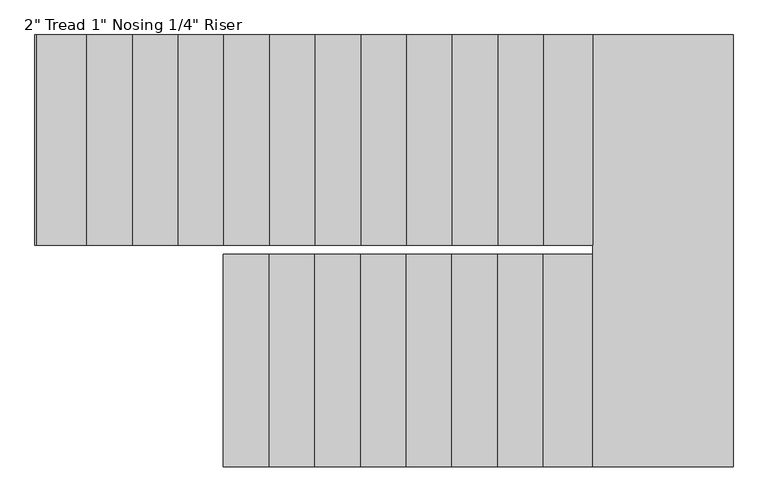
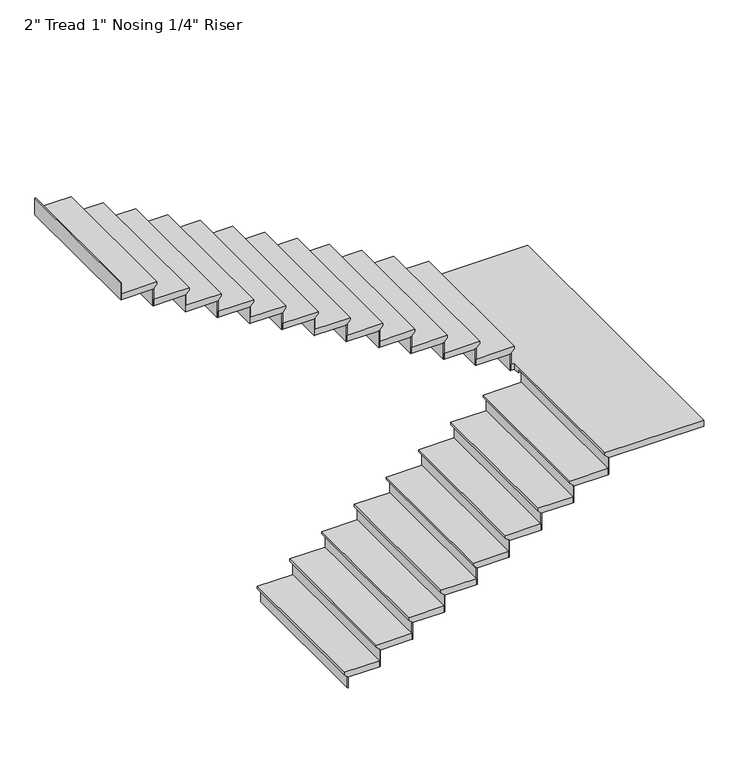
"""IFC4 building model written with IfcOpenShell, lengths in millimetres: stair flight geometry."""

from ifc_helpers import new_model, si_unit, origin, place, context, project, spatial, faceted_brep, source, transform, mapped, element, save


def stair_flight_9b376cb7(model_context):
    return source(origin(), model_context, "Body", "Brep", [
        faceted_brep([(2827.8890963, -935.5037749, 9263.4954545), (2827.8890963, -935.5037749, 9282.5454545), (2827.8890963, 245.5962251, 9282.5454545), (2827.8890963, 245.5962251, 9263.4954545), (2853.2890963, -935.5037749, 9238.0954545), (2853.2890963, 245.5962251, 9238.0954545), (3107.2890963, -935.5037749, 9282.5454545), (3107.2890963, 245.5962251, 9282.5454545), (2853.2890963, 245.5962251, 9231.7454545), (3107.2890963, 245.5962251, 9231.7454545), (3107.2890963, -935.5037749, 9231.7454545), (2853.2890963, -935.5037749, 9231.7454545)], [[[0, 1, 2, 3]], [[4, 0, 3, 5]], [[2, 1, 6, 7]], [[8, 9, 10, 11]], [[2, 7, 9, 8, 5, 3]], [[8, 11, 4, 5]], [[6, 1, 0, 4, 11, 10]], [[7, 6, 10, 9]]]),
        faceted_brep([(2853.2890963, -935.5037749, 9231.7454545), (2853.2890963, -935.5037749, 9144.0), (2859.6390963, -935.5037749, 9144.0), (2859.6390963, -935.5037749, 9231.7454545), (2853.2890963, 245.5962251, 9231.7454545), (2859.6390963, 245.5962251, 9231.7454545), (2859.6390963, 245.5962251, 9144.0), (2853.2890963, 245.5962251, 9144.0)], [[[0, 1, 2, 3]], [[4, 5, 6, 7]], [[1, 0, 4, 7]], [[2, 1, 7, 6]], [[3, 2, 6, 5]], [[0, 3, 5, 4]]]),
        faceted_brep([(3107.2890963, -935.5037749, 9370.2909091), (3107.2890963, -935.5037749, 9231.7454545), (3113.6390963, -935.5037749, 9231.7454545), (3113.6390963, -935.5037749, 9370.2909091), (3107.2890963, 245.5962251, 9370.2909091), (3113.6390963, 245.5962251, 9370.2909091), (3113.6390963, 245.5962251, 9231.7454545), (3107.2890963, 245.5962251, 9231.7454545)], [[[0, 1, 2, 3]], [[4, 5, 6, 7]], [[1, 0, 4, 7]], [[2, 1, 7, 6]], [[3, 2, 6, 5]], [[0, 3, 5, 4]]]),
        faceted_brep([(3081.8890963, 245.5962251, 9421.0909091), (3081.8890963, -935.5037749, 9421.0909091), (3361.2890963, -935.5037749, 9421.0909091), (3361.2890963, 245.5962251, 9421.0909091), (3107.2890963, 245.5962251, 9370.2909091), (3361.2890963, 245.5962251, 9370.2909091), (3361.2890963, -935.5037749, 9370.2909091), (3107.2890963, -935.5037749, 9370.2909091), (3107.2890963, 245.5962251, 9376.6409091), (3081.8890963, 245.5962251, 9402.0409091), (3107.2890963, -935.5037749, 9376.6409091), (3081.8890963, -935.5037749, 9402.0409091)], [[[0, 1, 2, 3]], [[4, 5, 6, 7]], [[0, 3, 5, 4, 8, 9]], [[4, 7, 10, 8]], [[2, 1, 11, 10, 7, 6]], [[3, 2, 6, 5]], [[11, 1, 0, 9]], [[10, 11, 9, 8]]]),
        faceted_brep([(3361.2890963, -935.5037749, 9508.8363636), (3361.2890963, -935.5037749, 9370.2909091), (3367.6390963, -935.5037749, 9370.2909091), (3367.6390963, -935.5037749, 9508.8363636), (3361.2890963, 245.5962251, 9508.8363636), (3367.6390963, 245.5962251, 9508.8363636), (3367.6390963, 245.5962251, 9370.2909091), (3361.2890963, 245.5962251, 9370.2909091)], [[[0, 1, 2, 3]], [[4, 5, 6, 7]], [[1, 0, 4, 7]], [[2, 1, 7, 6]], [[3, 2, 6, 5]], [[0, 3, 5, 4]]]),
        faceted_brep([(3335.8890963, 245.5962251, 9559.6363636), (3335.8890963, -935.5037749, 9559.6363636), (3615.2890963, -935.5037749, 9559.6363636), (3615.2890963, 245.5962251, 9559.6363636), (3361.2890963, 245.5962251, 9508.8363636), (3615.2890963, 245.5962251, 9508.8363636), (3615.2890963, -935.5037749, 9508.8363636), (3361.2890963, -935.5037749, 9508.8363636), (3361.2890963, 245.5962251, 9515.1863636), (3335.8890963, 245.5962251, 9540.5863636), (3361.2890963, -935.5037749, 9515.1863636), (3335.8890963, -935.5037749, 9540.5863636)], [[[0, 1, 2, 3]], [[4, 5, 6, 7]], [[0, 3, 5, 4, 8, 9]], [[4, 7, 10, 8]], [[2, 1, 11, 10, 7, 6]], [[3, 2, 6, 5]], [[11, 1, 0, 9]], [[10, 11, 9, 8]]]),
        faceted_brep([(3615.2890963, -935.5037749, 9647.3818182), (3615.2890963, -935.5037749, 9508.8363636), (3621.6390963, -935.5037749, 9508.8363636), (3621.6390963, -935.5037749, 9647.3818182), (3615.2890963, 245.5962251, 9647.3818182), (3621.6390963, 245.5962251, 9647.3818182), (3621.6390963, 245.5962251, 9508.8363636), (3615.2890963, 245.5962251, 9508.8363636)], [[[0, 1, 2, 3]], [[4, 5, 6, 7]], [[1, 0, 4, 7]], [[2, 1, 7, 6]], [[3, 2, 6, 5]], [[0, 3, 5, 4]]]),
        faceted_brep([(3589.8890963, 245.5962251, 9698.1818182), (3589.8890963, -935.5037749, 9698.1818182), (3869.2890963, -935.5037749, 9698.1818182), (3869.2890963, 245.5962251, 9698.1818182), (3615.2890963, 245.5962251, 9647.3818182), (3869.2890963, 245.5962251, 9647.3818182), (3869.2890963, -935.5037749, 9647.3818182), (3615.2890963, -935.5037749, 9647.3818182), (3615.2890963, 245.5962251, 9653.7318182), (3589.8890963, 245.5962251, 9679.1318182), (3615.2890963, -935.5037749, 9653.7318182), (3589.8890963, -935.5037749, 9679.1318182)], [[[0, 1, 2, 3]], [[4, 5, 6, 7]], [[0, 3, 5, 4, 8, 9]], [[4, 7, 10, 8]], [[2, 1, 11, 10, 7, 6]], [[3, 2, 6, 5]], [[11, 1, 0, 9]], [[10, 11, 9, 8]]]),
        faceted_brep([(3869.2890963, -935.5037749, 9785.9272727), (3869.2890963, -935.5037749, 9647.3818182), (3875.6390963, -935.5037749, 9647.3818182), (3875.6390963, -935.5037749, 9785.9272727), (3869.2890963, 245.5962251, 9785.9272727), (3875.6390963, 245.5962251, 9785.9272727), (3875.6390963, 245.5962251, 9647.3818182), (3869.2890963, 245.5962251, 9647.3818182)], [[[0, 1, 2, 3]], [[4, 5, 6, 7]], [[1, 0, 4, 7]], [[2, 1, 7, 6]], [[3, 2, 6, 5]], [[0, 3, 5, 4]]]),
        faceted_brep([(3843.8890963, 245.5962251, 9836.7272727), (3843.8890963, -935.5037749, 9836.7272727), (4123.2890963, -935.5037749, 9836.7272727), (4123.2890963, 245.5962251, 9836.7272727), (3869.2890963, 245.5962251, 9785.9272727), (4123.2890963, 245.5962251, 9785.9272727), (4123.2890963, -935.5037749, 9785.9272727), (3869.2890963, -935.5037749, 9785.9272727), (3869.2890963, 245.5962251, 9792.2772727), (3843.8890963, 245.5962251, 9817.6772727), (3869.2890963, -935.5037749, 9792.2772727), (3843.8890963, -935.5037749, 9817.6772727)], [[[0, 1, 2, 3]], [[4, 5, 6, 7]], [[0, 3, 5, 4, 8, 9]], [[4, 7, 10, 8]], [[2, 1, 11, 10, 7, 6]], [[3, 2, 6, 5]], [[11, 1, 0, 9]], [[10, 11, 9, 8]]]),
        faceted_brep([(4123.2890963, -935.5037749, 9924.4727273), (4123.2890963, -935.5037749, 9785.9272727), (4129.6390963, -935.5037749, 9785.9272727), (4129.6390963, -935.5037749, 9924.4727273), (4123.2890963, 245.5962251, 9924.4727273), (4129.6390963, 245.5962251, 9924.4727273), (4129.6390963, 245.5962251, 9785.9272727), (4123.2890963, 245.5962251, 9785.9272727)], [[[0, 1, 2, 3]], [[4, 5, 6, 7]], [[1, 0, 4, 7]], [[2, 1, 7, 6]], [[3, 2, 6, 5]], [[0, 3, 5, 4]]]),
        faceted_brep([(4097.8890963, 245.5962251, 9975.2727273), (4097.8890963, -935.5037749, 9975.2727273), (4377.2890963, -935.5037749, 9975.2727273), (4377.2890963, 245.5962251, 9975.2727273), (4123.2890963, 245.5962251, 9924.4727273), (4377.2890963, 245.5962251, 9924.4727273), (4377.2890963, -935.5037749, 9924.4727273), (4123.2890963, -935.5037749, 9924.4727273), (4123.2890963, 245.5962251, 9930.8227273), (4097.8890963, 245.5962251, 9956.2227273), (4123.2890963, -935.5037749, 9930.8227273), (4097.8890963, -935.5037749, 9956.2227273)], [[[0, 1, 2, 3]], [[4, 5, 6, 7]], [[0, 3, 5, 4, 8, 9]], [[4, 7, 10, 8]], [[2, 1, 11, 10, 7, 6]], [[3, 2, 6, 5]], [[11, 1, 0, 9]], [[10, 11, 9, 8]]]),
        faceted_brep([(4377.2890963, -935.5037749, 10063.0181818), (4377.2890963, -935.5037749, 9924.4727273), (4383.6390963, -935.5037749, 9924.4727273), (4383.6390963, -935.5037749, 10063.0181818), (4377.2890963, 245.5962251, 10063.0181818), (4383.6390963, 245.5962251, 10063.0181818), (4383.6390963, 245.5962251, 9924.4727273), (4377.2890963, 245.5962251, 9924.4727273)], [[[0, 1, 2, 3]], [[4, 5, 6, 7]], [[1, 0, 4, 7]], [[2, 1, 7, 6]], [[3, 2, 6, 5]], [[0, 3, 5, 4]]]),
        faceted_brep([(4351.8890963, 245.5962251, 10113.8181818), (4351.8890963, -935.5037749, 10113.8181818), (4631.2890963, -935.5037749, 10113.8181818), (4631.2890963, 245.5962251, 10113.8181818), (4377.2890963, 245.5962251, 10063.0181818), (4631.2890963, 245.5962251, 10063.0181818), (4631.2890963, -935.5037749, 10063.0181818), (4377.2890963, -935.5037749, 10063.0181818), (4377.2890963, 245.5962251, 10069.3681818), (4351.8890963, 245.5962251, 10094.7681818), (4377.2890963, -935.5037749, 10069.3681818), (4351.8890963, -935.5037749, 10094.7681818)], [[[0, 1, 2, 3]], [[4, 5, 6, 7]], [[0, 3, 5, 4, 8, 9]], [[4, 7, 10, 8]], [[2, 1, 11, 10, 7, 6]], [[3, 2, 6, 5]], [[11, 1, 0, 9]], [[10, 11, 9, 8]]]),
        faceted_brep([(1786.4890963, 1464.7962251, 12141.2), (1786.4890963, 1464.7962251, 12002.6545455), (1780.1390963, 1464.7962251, 12002.6545455), (1780.1390963, 1464.7962251, 12141.2), (1786.4890963, 296.3962251, 12141.2), (1780.1390963, 296.3962251, 12141.2), (1780.1390963, 296.3962251, 12002.6545455), (1786.4890963, 296.3962251, 12002.6545455)], [[[0, 1, 2, 3]], [[4, 5, 6, 7]], [[1, 0, 4, 7]], [[2, 1, 7, 6]], [[3, 2, 6, 5]], [[0, 3, 5, 4]]]),
        faceted_brep([(4631.2890963, -935.5037749, 10201.5636364), (4631.2890963, -935.5037749, 10063.0181818), (4637.6390963, -935.5037749, 10063.0181818), (4637.6390963, -935.5037749, 10201.5636364), (4631.2890963, 245.5962251, 10201.5636364), (4637.6390963, 245.5962251, 10201.5636364), (4637.6390963, 245.5962251, 10063.0181818), (4631.2890963, 245.5962251, 10063.0181818)], [[[0, 1, 2, 3]], [[4, 5, 6, 7]], [[1, 0, 4, 7]], [[2, 1, 7, 6]], [[3, 2, 6, 5]], [[0, 3, 5, 4]]]),
        faceted_brep([(4605.8890963, 245.5962251, 10252.3636364), (4605.8890963, -935.5037749, 10252.3636364), (4906.4326586, -935.5037749, 10252.3636364), (4906.4326586, 245.5962251, 10252.3636364), (4631.2890963, 245.5962251, 10201.5636364), (4906.4326586, 245.5962251, 10201.5636364), (4906.4326586, -935.5037749, 10201.5636364), (4631.2890963, -935.5037749, 10201.5636364), (4631.2890963, 245.5962251, 10207.9136364), (4605.8890963, 245.5962251, 10233.3136364), (4631.2890963, -935.5037749, 10207.9136364), (4605.8890963, -935.5037749, 10233.3136364)], [[[0, 1, 2, 3]], [[4, 5, 6, 7]], [[0, 3, 5, 4, 8, 9]], [[4, 7, 10, 8]], [[2, 1, 11, 10, 7, 6]], [[3, 2, 6, 5]], [[11, 1, 0, 9]], [[10, 11, 9, 8]]]),
        faceted_brep([(4906.4326586, -935.5037749, 10340.1090909), (4906.4326586, -935.5037749, 10201.5636364), (4912.7826586, -935.5037749, 10201.5636364), (4912.7826586, -935.5037749, 10340.1090909), (4906.4326586, 245.5962251, 10340.1090909), (4912.7826586, 245.5962251, 10340.1090909), (4912.7826586, 245.5962251, 10201.5636364), (4906.4326586, 245.5962251, 10201.5636364)], [[[0, 1, 2, 3]], [[4, 5, 6, 7]], [[1, 0, 4, 7]], [[2, 1, 7, 6]], [[3, 2, 6, 5]], [[0, 3, 5, 4]]]),
        faceted_brep([(4855.6326586, 296.3962251, 10390.9090909), (4881.0326586, 296.3962251, 10390.9090909), (4881.0326586, -935.5037749, 10390.9090909), (5659.9890963, -935.5037749, 10390.9090909), (5659.9890963, 1464.7962251, 10390.9090909), (4855.6326586, 1464.7962251, 10390.9090909), (4881.0326586, 296.3962251, 10340.1090909), (4855.6326586, 296.3962251, 10340.1090909), (4855.6326586, 1464.7962251, 10340.1090909), (5659.9890963, 1464.7962251, 10340.1090909), (5659.9890963, -935.5037749, 10340.1090909), (4906.4326586, -935.5037749, 10340.1090909), (4906.4326586, 245.5962251, 10340.1090909), (4881.0326586, 245.5962251, 10340.1090909), (4881.0326586, 245.5962251, 10371.8590909), (4881.0326586, -935.5037749, 10371.8590909), (4906.4326586, 245.5962251, 10346.4590909), (4906.4326586, -935.5037749, 10346.4590909)], [[[0, 1, 2, 3, 4, 5]], [[6, 7, 8, 9, 10, 11, 12, 13]], [[1, 0, 7, 6]], [[2, 1, 6, 13, 14, 15]], [[13, 12, 16, 14]], [[12, 11, 17, 16]], [[3, 2, 15, 17, 11, 10]], [[4, 3, 10, 9]], [[5, 4, 9, 8]], [[0, 5, 8, 7]], [[17, 15, 14, 16]]]),
        faceted_brep([(4855.6326586, 1464.7962251, 10478.6545455), (4855.6326586, 1464.7962251, 10340.1090909), (4849.2826586, 1464.7962251, 10340.1090909), (4849.2826586, 1464.7962251, 10478.6545455), (4855.6326586, 296.3962251, 10478.6545455), (4849.2826586, 296.3962251, 10478.6545455), (4849.2826586, 296.3962251, 10340.1090909), (4855.6326586, 296.3962251, 10340.1090909)], [[[0, 1, 2, 3]], [[4, 5, 6, 7]], [[1, 0, 4, 7]], [[2, 1, 7, 6]], [[3, 2, 6, 5]], [[0, 3, 5, 4]]]),
        faceted_brep([(4881.0326586, 296.3962251, 10529.4545455), (4881.0326586, 1464.7962251, 10529.4545455), (4580.4890963, 1464.7962251, 10529.4545455), (4580.4890963, 296.3962251, 10529.4545455), (4855.6326586, 296.3962251, 10478.6545455), (4580.4890963, 296.3962251, 10478.6545455), (4580.4890963, 1464.7962251, 10478.6545455), (4855.6326586, 1464.7962251, 10478.6545455), (4855.6326586, 296.3962251, 10485.0045455), (4881.0326586, 296.3962251, 10510.4045455), (4855.6326586, 1464.7962251, 10485.0045455), (4881.0326586, 1464.7962251, 10510.4045455)], [[[0, 1, 2, 3]], [[4, 5, 6, 7]], [[0, 3, 5, 4, 8, 9]], [[4, 7, 10, 8]], [[2, 1, 11, 10, 7, 6]], [[3, 2, 6, 5]], [[11, 1, 0, 9]], [[10, 11, 9, 8]]]),
        faceted_brep([(4580.4890963, 1464.7962251, 10617.2), (4580.4890963, 1464.7962251, 10478.6545455), (4574.1390963, 1464.7962251, 10478.6545455), (4574.1390963, 1464.7962251, 10617.2), (4580.4890963, 296.3962251, 10617.2), (4574.1390963, 296.3962251, 10617.2), (4574.1390963, 296.3962251, 10478.6545455), (4580.4890963, 296.3962251, 10478.6545455)], [[[0, 1, 2, 3]], [[4, 5, 6, 7]], [[1, 0, 4, 7]], [[2, 1, 7, 6]], [[3, 2, 6, 5]], [[0, 3, 5, 4]]]),
        faceted_brep([(4605.8890963, 296.3962251, 10668.0), (4605.8890963, 1464.7962251, 10668.0), (4326.4890963, 1464.7962251, 10668.0), (4326.4890963, 296.3962251, 10668.0), (4580.4890963, 296.3962251, 10617.2), (4326.4890963, 296.3962251, 10617.2), (4326.4890963, 1464.7962251, 10617.2), (4580.4890963, 1464.7962251, 10617.2), (4580.4890963, 296.3962251, 10623.55), (4605.8890963, 296.3962251, 10648.95), (4580.4890963, 1464.7962251, 10623.55), (4605.8890963, 1464.7962251, 10648.95)], [[[0, 1, 2, 3]], [[4, 5, 6, 7]], [[0, 3, 5, 4, 8, 9]], [[4, 7, 10, 8]], [[2, 1, 11, 10, 7, 6]], [[3, 2, 6, 5]], [[11, 1, 0, 9]], [[10, 11, 9, 8]]]),
        faceted_brep([(4326.4890963, 1464.7962251, 10755.7454545), (4326.4890963, 1464.7962251, 10617.2), (4320.1390963, 1464.7962251, 10617.2), (4320.1390963, 1464.7962251, 10755.7454545), (4326.4890963, 296.3962251, 10755.7454545), (4320.1390963, 296.3962251, 10755.7454545), (4320.1390963, 296.3962251, 10617.2), (4326.4890963, 296.3962251, 10617.2)], [[[0, 1, 2, 3]], [[4, 5, 6, 7]], [[1, 0, 4, 7]], [[2, 1, 7, 6]], [[3, 2, 6, 5]], [[0, 3, 5, 4]]]),
        faceted_brep([(4351.8890963, 296.3962251, 10806.5454545), (4351.8890963, 1464.7962251, 10806.5454545), (4072.4890963, 1464.7962251, 10806.5454545), (4072.4890963, 296.3962251, 10806.5454545), (4326.4890963, 296.3962251, 10755.7454545), (4072.4890963, 296.3962251, 10755.7454545), (4072.4890963, 1464.7962251, 10755.7454545), (4326.4890963, 1464.7962251, 10755.7454545), (4326.4890963, 296.3962251, 10762.0954545), (4351.8890963, 296.3962251, 10787.4954545), (4326.4890963, 1464.7962251, 10762.0954545), (4351.8890963, 1464.7962251, 10787.4954545)], [[[0, 1, 2, 3]], [[4, 5, 6, 7]], [[0, 3, 5, 4, 8, 9]], [[4, 7, 10, 8]], [[2, 1, 11, 10, 7, 6]], [[3, 2, 6, 5]], [[11, 1, 0, 9]], [[10, 11, 9, 8]]]),
        faceted_brep([(4072.4890963, 1464.7962251, 10894.2909091), (4072.4890963, 1464.7962251, 10755.7454545), (4066.1390963, 1464.7962251, 10755.7454545), (4066.1390963, 1464.7962251, 10894.2909091), (4072.4890963, 296.3962251, 10894.2909091), (4066.1390963, 296.3962251, 10894.2909091), (4066.1390963, 296.3962251, 10755.7454545), (4072.4890963, 296.3962251, 10755.7454545)], [[[0, 1, 2, 3]], [[4, 5, 6, 7]], [[1, 0, 4, 7]], [[2, 1, 7, 6]], [[3, 2, 6, 5]], [[0, 3, 5, 4]]]),
        faceted_brep([(4097.8890963, 296.3962251, 10945.0909091), (4097.8890963, 1464.7962251, 10945.0909091), (3818.4890963, 1464.7962251, 10945.0909091), (3818.4890963, 296.3962251, 10945.0909091), (4072.4890963, 296.3962251, 10894.2909091), (3818.4890963, 296.3962251, 10894.2909091), (3818.4890963, 1464.7962251, 10894.2909091), (4072.4890963, 1464.7962251, 10894.2909091), (4072.4890963, 296.3962251, 10900.6409091), (4097.8890963, 296.3962251, 10926.0409091), (4072.4890963, 1464.7962251, 10900.6409091), (4097.8890963, 1464.7962251, 10926.0409091)], [[[0, 1, 2, 3]], [[4, 5, 6, 7]], [[0, 3, 5, 4, 8, 9]], [[4, 7, 10, 8]], [[2, 1, 11, 10, 7, 6]], [[3, 2, 6, 5]], [[11, 1, 0, 9]], [[10, 11, 9, 8]]]),
        faceted_brep([(3818.4890963, 1464.7962251, 11032.8363636), (3818.4890963, 1464.7962251, 10894.2909091), (3812.1390963, 1464.7962251, 10894.2909091), (3812.1390963, 1464.7962251, 11032.8363636), (3818.4890963, 296.3962251, 11032.8363636), (3812.1390963, 296.3962251, 11032.8363636), (3812.1390963, 296.3962251, 10894.2909091), (3818.4890963, 296.3962251, 10894.2909091)], [[[0, 1, 2, 3]], [[4, 5, 6, 7]], [[1, 0, 4, 7]], [[2, 1, 7, 6]], [[3, 2, 6, 5]], [[0, 3, 5, 4]]]),
        faceted_brep([(3843.8890963, 296.3962251, 11083.6363636), (3843.8890963, 1464.7962251, 11083.6363636), (3564.4890963, 1464.7962251, 11083.6363636), (3564.4890963, 296.3962251, 11083.6363636), (3818.4890963, 296.3962251, 11032.8363636), (3564.4890963, 296.3962251, 11032.8363636), (3564.4890963, 1464.7962251, 11032.8363636), (3818.4890963, 1464.7962251, 11032.8363636), (3818.4890963, 296.3962251, 11039.1863636), (3843.8890963, 296.3962251, 11064.5863636), (3818.4890963, 1464.7962251, 11039.1863636), (3843.8890963, 1464.7962251, 11064.5863636)], [[[0, 1, 2, 3]], [[4, 5, 6, 7]], [[0, 3, 5, 4, 8, 9]], [[4, 7, 10, 8]], [[2, 1, 11, 10, 7, 6]], [[3, 2, 6, 5]], [[11, 1, 0, 9]], [[10, 11, 9, 8]]]),
        faceted_brep([(3564.4890963, 1464.7962251, 11171.3818182), (3564.4890963, 1464.7962251, 11032.8363636), (3558.1390963, 1464.7962251, 11032.8363636), (3558.1390963, 1464.7962251, 11171.3818182), (3564.4890963, 296.3962251, 11171.3818182), (3558.1390963, 296.3962251, 11171.3818182), (3558.1390963, 296.3962251, 11032.8363636), (3564.4890963, 296.3962251, 11032.8363636)], [[[0, 1, 2, 3]], [[4, 5, 6, 7]], [[1, 0, 4, 7]], [[2, 1, 7, 6]], [[3, 2, 6, 5]], [[0, 3, 5, 4]]]),
        faceted_brep([(3589.8890963, 296.3962251, 11222.1818182), (3589.8890963, 1464.7962251, 11222.1818182), (3310.4890963, 1464.7962251, 11222.1818182), (3310.4890963, 296.3962251, 11222.1818182), (3564.4890963, 296.3962251, 11171.3818182), (3310.4890963, 296.3962251, 11171.3818182), (3310.4890963, 1464.7962251, 11171.3818182), (3564.4890963, 1464.7962251, 11171.3818182), (3564.4890963, 296.3962251, 11177.7318182), (3589.8890963, 296.3962251, 11203.1318182), (3564.4890963, 1464.7962251, 11177.7318182), (3589.8890963, 1464.7962251, 11203.1318182)], [[[0, 1, 2, 3]], [[4, 5, 6, 7]], [[0, 3, 5, 4, 8, 9]], [[4, 7, 10, 8]], [[2, 1, 11, 10, 7, 6]], [[3, 2, 6, 5]], [[11, 1, 0, 9]], [[10, 11, 9, 8]]]),
        faceted_brep([(3310.4890963, 1464.7962251, 11309.9272727), (3310.4890963, 1464.7962251, 11171.3818182), (3304.1390963, 1464.7962251, 11171.3818182), (3304.1390963, 1464.7962251, 11309.9272727), (3310.4890963, 296.3962251, 11309.9272727), (3304.1390963, 296.3962251, 11309.9272727), (3304.1390963, 296.3962251, 11171.3818182), (3310.4890963, 296.3962251, 11171.3818182)], [[[0, 1, 2, 3]], [[4, 5, 6, 7]], [[1, 0, 4, 7]], [[2, 1, 7, 6]], [[3, 2, 6, 5]], [[0, 3, 5, 4]]]),
        faceted_brep([(3335.8890963, 296.3962251, 11360.7272727), (3335.8890963, 1464.7962251, 11360.7272727), (3056.4890963, 1464.7962251, 11360.7272727), (3056.4890963, 296.3962251, 11360.7272727), (3310.4890963, 296.3962251, 11309.9272727), (3056.4890963, 296.3962251, 11309.9272727), (3056.4890963, 1464.7962251, 11309.9272727), (3310.4890963, 1464.7962251, 11309.9272727), (3310.4890963, 296.3962251, 11316.2772727), (3335.8890963, 296.3962251, 11341.6772727), (3310.4890963, 1464.7962251, 11316.2772727), (3335.8890963, 1464.7962251, 11341.6772727)], [[[0, 1, 2, 3]], [[4, 5, 6, 7]], [[0, 3, 5, 4, 8, 9]], [[4, 7, 10, 8]], [[2, 1, 11, 10, 7, 6]], [[3, 2, 6, 5]], [[11, 1, 0, 9]], [[10, 11, 9, 8]]]),
        faceted_brep([(3056.4890963, 1464.7962251, 11448.4727273), (3056.4890963, 1464.7962251, 11309.9272727), (3050.1390963, 1464.7962251, 11309.9272727), (3050.1390963, 1464.7962251, 11448.4727273), (3056.4890963, 296.3962251, 11448.4727273), (3050.1390963, 296.3962251, 11448.4727273), (3050.1390963, 296.3962251, 11309.9272727), (3056.4890963, 296.3962251, 11309.9272727)], [[[0, 1, 2, 3]], [[4, 5, 6, 7]], [[1, 0, 4, 7]], [[2, 1, 7, 6]], [[3, 2, 6, 5]], [[0, 3, 5, 4]]]),
        faceted_brep([(3081.8890963, 296.3962251, 11499.2727273), (3081.8890963, 1464.7962251, 11499.2727273), (2802.4890963, 1464.7962251, 11499.2727273), (2802.4890963, 296.3962251, 11499.2727273), (3056.4890963, 296.3962251, 11448.4727273), (2802.4890963, 296.3962251, 11448.4727273), (2802.4890963, 1464.7962251, 11448.4727273), (3056.4890963, 1464.7962251, 11448.4727273), (3056.4890963, 296.3962251, 11454.8227273), (3081.8890963, 296.3962251, 11480.2227273), (3056.4890963, 1464.7962251, 11454.8227273), (3081.8890963, 1464.7962251, 11480.2227273)], [[[0, 1, 2, 3]], [[4, 5, 6, 7]], [[0, 3, 5, 4, 8, 9]], [[4, 7, 10, 8]], [[2, 1, 11, 10, 7, 6]], [[3, 2, 6, 5]], [[11, 1, 0, 9]], [[10, 11, 9, 8]]]),
        faceted_brep([(2802.4890963, 1464.7962251, 11587.0181818), (2802.4890963, 1464.7962251, 11448.4727273), (2796.1390963, 1464.7962251, 11448.4727273), (2796.1390963, 1464.7962251, 11587.0181818), (2802.4890963, 296.3962251, 11587.0181818), (2796.1390963, 296.3962251, 11587.0181818), (2796.1390963, 296.3962251, 11448.4727273), (2802.4890963, 296.3962251, 11448.4727273)], [[[0, 1, 2, 3]], [[4, 5, 6, 7]], [[1, 0, 4, 7]], [[2, 1, 7, 6]], [[3, 2, 6, 5]], [[0, 3, 5, 4]]]),
        faceted_brep([(2827.8890963, 296.3962251, 11637.8181818), (2827.8890963, 1464.7962251, 11637.8181818), (2548.4890963, 1464.7962251, 11637.8181818), (2548.4890963, 296.3962251, 11637.8181818), (2802.4890963, 296.3962251, 11587.0181818), (2548.4890963, 296.3962251, 11587.0181818), (2548.4890963, 1464.7962251, 11587.0181818), (2802.4890963, 1464.7962251, 11587.0181818), (2802.4890963, 296.3962251, 11593.3681818), (2827.8890963, 296.3962251, 11618.7681818), (2802.4890963, 1464.7962251, 11593.3681818), (2827.8890963, 1464.7962251, 11618.7681818)], [[[0, 1, 2, 3]], [[4, 5, 6, 7]], [[0, 3, 5, 4, 8, 9]], [[4, 7, 10, 8]], [[2, 1, 11, 10, 7, 6]], [[3, 2, 6, 5]], [[11, 1, 0, 9]], [[10, 11, 9, 8]]]),
        faceted_brep([(2548.4890963, 1464.7962251, 11725.5636364), (2548.4890963, 1464.7962251, 11587.0181818), (2542.1390963, 1464.7962251, 11587.0181818), (2542.1390963, 1464.7962251, 11725.5636364), (2548.4890963, 296.3962251, 11725.5636364), (2542.1390963, 296.3962251, 11725.5636364), (2542.1390963, 296.3962251, 11587.0181818), (2548.4890963, 296.3962251, 11587.0181818)], [[[0, 1, 2, 3]], [[4, 5, 6, 7]], [[1, 0, 4, 7]], [[2, 1, 7, 6]], [[3, 2, 6, 5]], [[0, 3, 5, 4]]]),
        faceted_brep([(2573.8890963, 296.3962251, 11776.3636364), (2573.8890963, 1464.7962251, 11776.3636364), (2294.4890963, 1464.7962251, 11776.3636364), (2294.4890963, 296.3962251, 11776.3636364), (2548.4890963, 296.3962251, 11725.5636364), (2294.4890963, 296.3962251, 11725.5636364), (2294.4890963, 1464.7962251, 11725.5636364), (2548.4890963, 1464.7962251, 11725.5636364), (2548.4890963, 296.3962251, 11731.9136364), (2573.8890963, 296.3962251, 11757.3136364), (2548.4890963, 1464.7962251, 11731.9136364), (2573.8890963, 1464.7962251, 11757.3136364)], [[[0, 1, 2, 3]], [[4, 5, 6, 7]], [[0, 3, 5, 4, 8, 9]], [[4, 7, 10, 8]], [[2, 1, 11, 10, 7, 6]], [[3, 2, 6, 5]], [[11, 1, 0, 9]], [[10, 11, 9, 8]]]),
        faceted_brep([(2294.4890963, 1464.7962251, 11864.1090909), (2294.4890963, 1464.7962251, 11725.5636364), (2288.1390963, 1464.7962251, 11725.5636364), (2288.1390963, 1464.7962251, 11864.1090909), (2294.4890963, 296.3962251, 11864.1090909), (2288.1390963, 296.3962251, 11864.1090909), (2288.1390963, 296.3962251, 11725.5636364), (2294.4890963, 296.3962251, 11725.5636364)], [[[0, 1, 2, 3]], [[4, 5, 6, 7]], [[1, 0, 4, 7]], [[2, 1, 7, 6]], [[3, 2, 6, 5]], [[0, 3, 5, 4]]]),
        faceted_brep([(2319.8890963, 296.3962251, 11914.9090909), (2319.8890963, 1464.7962251, 11914.9090909), (2040.4890963, 1464.7962251, 11914.9090909), (2040.4890963, 296.3962251, 11914.9090909), (2294.4890963, 296.3962251, 11864.1090909), (2040.4890963, 296.3962251, 11864.1090909), (2040.4890963, 1464.7962251, 11864.1090909), (2294.4890963, 1464.7962251, 11864.1090909), (2294.4890963, 296.3962251, 11870.4590909), (2319.8890963, 296.3962251, 11895.8590909), (2294.4890963, 1464.7962251, 11870.4590909), (2319.8890963, 1464.7962251, 11895.8590909)], [[[0, 1, 2, 3]], [[4, 5, 6, 7]], [[0, 3, 5, 4, 8, 9]], [[4, 7, 10, 8]], [[2, 1, 11, 10, 7, 6]], [[3, 2, 6, 5]], [[11, 1, 0, 9]], [[10, 11, 9, 8]]]),
        faceted_brep([(2040.4890963, 1464.7962251, 12002.6545455), (2040.4890963, 1464.7962251, 11864.1090909), (2034.1390963, 1464.7962251, 11864.1090909), (2034.1390963, 1464.7962251, 12002.6545455), (2040.4890963, 296.3962251, 12002.6545455), (2034.1390963, 296.3962251, 12002.6545455), (2034.1390963, 296.3962251, 11864.1090909), (2040.4890963, 296.3962251, 11864.1090909)], [[[0, 1, 2, 3]], [[4, 5, 6, 7]], [[1, 0, 4, 7]], [[2, 1, 7, 6]], [[3, 2, 6, 5]], [[0, 3, 5, 4]]]),
        faceted_brep([(2065.8890963, 296.3962251, 12053.4545455), (2065.8890963, 1464.7962251, 12053.4545455), (1786.4890963, 1464.7962251, 12053.4545455), (1786.4890963, 296.3962251, 12053.4545455), (2040.4890963, 296.3962251, 12002.6545455), (1786.4890963, 296.3962251, 12002.6545455), (1786.4890963, 1464.7962251, 12002.6545455), (2040.4890963, 1464.7962251, 12002.6545455), (2040.4890963, 296.3962251, 12009.0045455), (2065.8890963, 296.3962251, 12034.4045455), (2040.4890963, 1464.7962251, 12009.0045455), (2065.8890963, 1464.7962251, 12034.4045455)], [[[0, 1, 2, 3]], [[4, 5, 6, 7]], [[0, 3, 5, 4, 8, 9]], [[4, 7, 10, 8]], [[2, 1, 11, 10, 7, 6]], [[3, 2, 6, 5]], [[11, 1, 0, 9]], [[10, 11, 9, 8]]]),
    ])


if __name__ == "__main__":
    model = new_model("IFC4")
    model_context = context("Model", 3, world=origin())
    ifc_project = project(units=[si_unit("LENGTHUNIT", "METRE", prefix="MILLI")], contexts=[model_context])
    site = spatial("IfcSite", under=ifc_project)
    building = spatial("IfcBuilding", under=site)
    placement = place(None, origin())
    stair_flight_shape = stair_flight_9b376cb7(model_context)
    element("IfcStairFlight", 1, ObjectType="2\" Tread 1\" Nosing 1/4\" Riser", at=placement, inside=building, context=model_context, shape_type="MappedRepresentation", body=[
        mapped(stair_flight_shape, transform((0.0, 0.0, 0.0), x_axis=(1.0, 0.0, 0.0), y_axis=(0.0, 1.0, 0.0), z_axis=(0.0, 0.0, 1.0))),
    ])
    save(model, "model.ifc")
